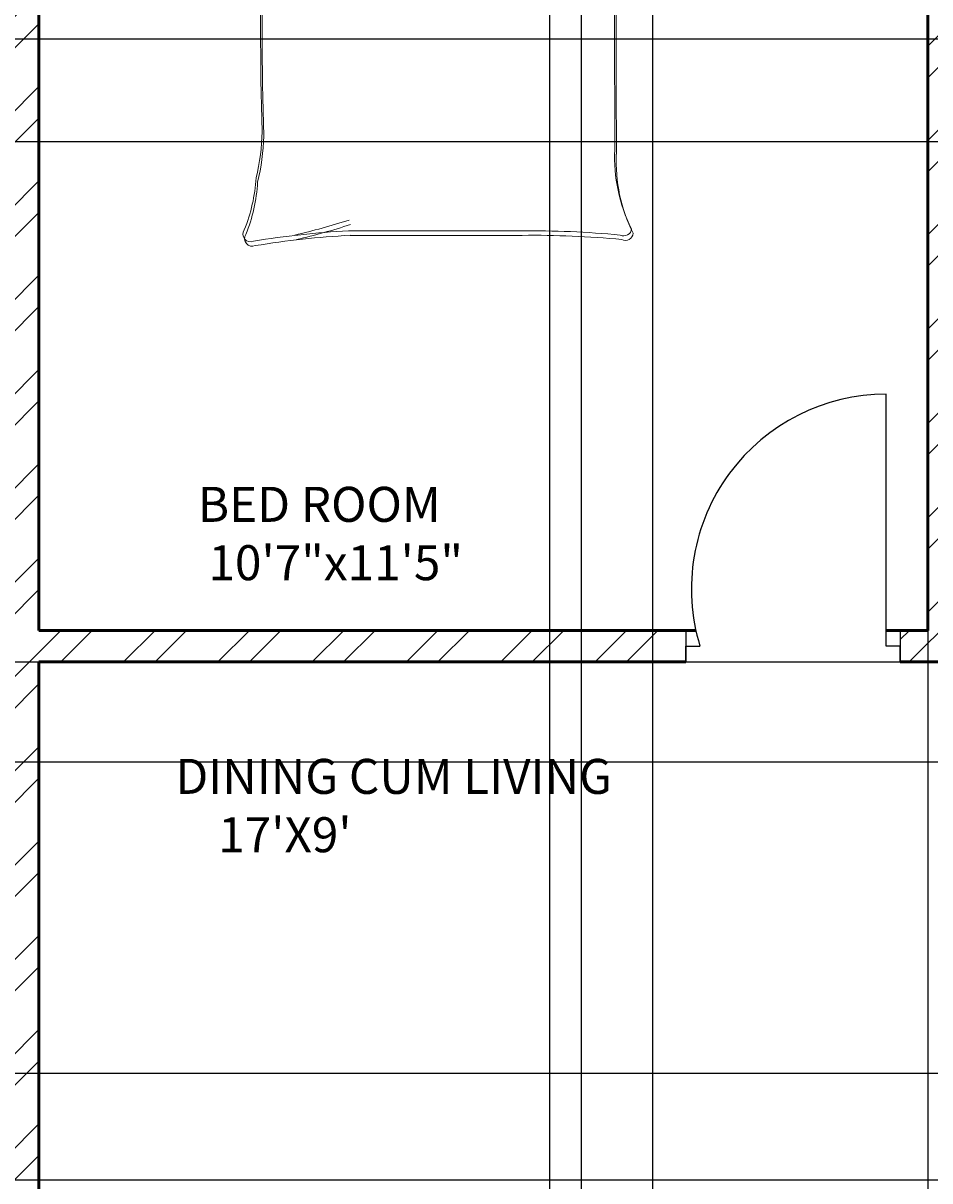
# Model space of a CAD drawing. Units: inches. Extents: x 2310 to 2937, y 1113 to 2410.
# Tile 20 of 23: x 2609 to 2739, y 2132 to 2297. Entities that reach past the tile are written whole.
import ezdxf

# ---------------------------------------------------------------- set-up
doc = ezdxf.new("R2010")
doc.units = ezdxf.units.IN
for name, color, linetype, lineweight in [('A-ANNO-DIMS', 2, 'Continuous', 18), ('A-AREA-IDEN', 7, 'Continuous', 18), ('A-DOOR', 31, 'Continuous', 25), ('A-FURN', 8, 'Continuous', 18), ('A-WALL', 7, 'Continuous', 50), ('A-WALL-PATT', 85, 'Continuous', 13)]:
    doc.layers.add(name, color=color, linetype=linetype, lineweight=lineweight)
doc.styles.get("Standard").update_dxf_attribs({"font": 'arial.ttf'})
doc.dimstyles.get("Standard").update_dxf_attribs({"dimtxt": 0.18, "dimasz": 0.18, "dimexe": 0.18, "dimexo": 0.0625, "dimgap": 0.09, "dimtad": 0, "dimtih": 1, "dimtoh": 1, "dimdec": 4, "dimzin": 0, "dimdsep": 46, "dimtxsty": 'Standard', "dimcen": 0.09, "dimadec": 0, "dimazin": 0, "dimtfac": 1, "dimtdec": 4, "dimtofl": 0, "dimtmove": 0, "dimatfit": 3, "dimfxl": 1, "dimtolj": 1, "dimtzin": 0, "dimarcsym": 0})

# ---------------------------------------------------------------- blocks, each defined once
blk = doc.blocks.new('BED-DOUBLE')
for p, q in [((3.56, 63.44), (3.56, 81.55)), ((3.56, 63.44), (3.56, 81.55)), ((3.56, 81.55), (51.58, 81.55)), ((51.35, 81.55), (51.35, 54.94)), ((51.35, 81.55), (51.35, 54.94)), ((51.58, 81.55), (51.58, 80.91)), ((3.56, 80.01), (51.35, 80.01)), ((3.56, 80.01), (51.35, 80.01)), ((3.79, 62.8), (3.79, 80.91)), ((3.79, 62.8), (3.79, 80.91)), ((24.62, 79.1), (26.07, 79.68)), ((24.62, 79.1), (26.07, 79.68)), ((26.07, 79.68), (26.65, 74.33)), ((26.07, 79.68), (26.65, 74.33)), ((51.58, 80.91), (51.58, 54.3)), ((51.58, 80.91), (51.58, 54.3)), ((3.79, 79.38), (51.58, 79.38)), ((3.79, 79.38), (51.58, 79.38)), ((3.98, 78.21), (8.27, 78.54)), ((3.98, 78.23), (4.56, 75.05)), ((3.98, 78.23), (4.56, 75.05)), ((3.99, 78.21), (8.27, 78.54)), ((4.21, 77.57), (8.49, 77.9)), ((4.21, 77.57), (8.49, 77.9)), ((8.27, 78.54), (8.37, 78.52)), ((8.27, 78.54), (8.37, 78.52)), ((8.37, 78.52), (12.19, 78.23)), ((8.37, 78.52), (12.19, 78.23)), ((8.49, 77.9), (8.6, 77.88)), ((8.49, 77.9), (8.6, 77.88)), ((8.6, 77.88), (12.42, 77.59)), ((8.6, 77.88), (12.42, 77.59)), ((12.19, 78.23), (17.69, 77.22)), ((12.19, 78.23), (17.69, 77.22)), ((14.94, 77.8), (16.97, 78.52)), ((14.94, 77.8), (16.96, 78.52)), ((15.17, 77.16), (17.19, 77.88)), ((15.17, 77.16), (17.19, 77.88)), ((16.96, 78.52), (19.86, 79.24)), ((16.97, 78.52), (19.86, 79.24)), ((17.19, 77.88), (20.08, 78.61)), ((17.19, 77.88), (20.08, 78.61)), ((19.86, 79.24), (20.18, 79.24)), ((19.86, 79.24), (20.18, 79.24)), ((20.08, 78.61), (20.41, 78.61)), ((20.08, 78.61), (20.41, 78.61)), ((20.18, 79.24), (24.62, 79.1)), ((20.18, 79.24), (24.62, 79.1)), ((20.41, 78.61), (24.85, 78.46)), ((20.41, 78.61), (24.85, 78.46)), ((24.85, 78.46), (26.3, 79.04)), ((24.85, 78.46), (26.3, 79.04)), ((26.3, 79.04), (26.88, 73.69)), ((26.3, 79.04), (26.88, 73.69)), ((28.06, 79.06), (27.82, 73.68)), ((28.06, 79.06), (27.82, 73.68)), ((28.29, 78.42), (28.05, 73.04)), ((28.29, 78.42), (28.05, 73.04)), ((29.54, 78.57), (28.06, 79.06)), ((29.54, 78.57), (28.06, 79.06)), ((29.77, 77.93), (28.29, 78.42)), ((29.77, 77.93), (28.29, 78.42)), ((33.97, 78.99), (29.54, 78.57)), ((33.97, 78.99), (29.54, 78.57)), ((34.2, 78.35), (29.77, 77.93)), ((34.2, 78.35), (29.77, 77.93)), ((34.29, 79.01), (33.97, 78.99)), ((34.29, 79.01), (33.97, 78.99)), ((34.52, 78.37), (34.2, 78.35)), ((34.52, 78.37), (34.2, 78.35)), ((37.22, 78.47), (34.29, 79.01)), ((37.22, 78.47), (34.29, 79.01)), ((37.45, 77.83), (34.52, 78.37)), ((37.45, 77.83), (34.52, 78.37)), ((42, 78.48), (36.58, 77.13)), ((42, 78.48), (36.58, 77.13)), ((42.23, 77.84), (36.81, 76.49)), ((42.23, 77.84), (36.81, 76.49)), ((39.29, 77.87), (37.22, 78.47)), ((39.29, 77.87), (37.22, 78.47)), ((39.52, 77.24), (37.45, 77.83)), ((39.51, 77.24), (37.45, 77.83)), ((45.8, 79.01), (42, 78.48)), ((45.8, 79.01), (42, 78.48)), ((46.03, 78.37), (42.23, 77.84)), ((46.03, 78.37), (42.23, 77.84)), ((50.2, 78.99), (44.8, 79.09)), ((44.8, 79.09), (45.8, 79.01)), ((50.2, 78.99), (44.8, 79.09)), ((44.8, 79.09), (45.8, 79.01)), ((50.43, 78.35), (45.02, 78.45)), ((45.02, 78.45), (46.03, 78.37)), ((50.43, 78.35), (45.02, 78.45)), ((45.02, 78.45), (46.03, 78.37)), ((50.2, 78.99), (49.82, 75.78)), ((50.2, 78.99), (49.82, 75.78)), ((50.43, 78.35), (50.05, 75.14)), ((50.43, 78.35), (50.05, 75.14)), ((4.21, 77.59), (4.79, 74.41)), ((4.21, 77.59), (4.79, 74.41)), ((12.42, 77.59), (17.92, 76.58)), ((12.42, 77.59), (17.92, 76.58)), ((4.56, 75.05), (4.13, 72.45)), ((4.56, 75.05), (4.13, 72.45)), ((5.14, 72.59), (6.15, 75.34)), ((5.14, 72.59), (6.15, 75.34)), ((5.37, 71.95), (6.38, 74.7)), ((5.37, 71.95), (6.38, 74.7)), ((49.4, 73.29), (48.21, 75.97)), ((49.4, 73.29), (48.21, 75.97)), ((49.62, 72.65), (48.44, 75.33)), ((49.62, 72.65), (48.44, 75.33)), ((49.82, 75.78), (50.42, 73.21)), ((49.82, 75.78), (50.41, 73.21)), ((50.05, 75.14), (50.64, 72.57)), ((50.05, 75.14), (50.64, 72.57)), ((4.79, 74.41), (4.35, 71.81)), ((4.79, 74.41), (4.35, 71.81)), ((26.65, 74.33), (27.23, 71.15)), ((26.65, 74.33), (27.23, 71.15)), ((26.88, 73.69), (27.45, 70.51)), ((26.88, 73.69), (27.45, 70.51)), ((27.82, 73.68), (27.44, 70.47)), ((27.82, 73.68), (27.44, 70.47)), ((28.05, 73.04), (27.67, 69.83)), ((28.05, 73.04), (27.67, 69.83)), ((50.2, 69.72), (49.4, 73.29)), ((50.2, 69.72), (49.4, 73.29)), ((50.42, 73.21), (49.9, 72.16)), ((50.41, 73.21), (49.9, 72.16)), ((4.13, 72.45), (4.7, 71.44)), ((4.13, 72.45), (4.7, 71.44)), ((4.35, 71.81), (4.93, 70.8)), ((4.35, 71.81), (4.93, 70.8)), ((4.56, 68.98), (5.14, 72.59)), ((4.56, 68.98), (5.14, 72.59)), ((4.79, 68.34), (5.37, 71.95)), ((4.79, 68.34), (5.37, 71.95)), ((27.23, 71.15), (27.23, 69.85)), ((27.23, 71.15), (27.23, 69.85)), ((50.43, 69.08), (49.62, 72.65)), ((50.43, 69.08), (49.62, 72.65)), ((50.64, 72.57), (50.13, 71.52)), ((50.64, 72.57), (50.13, 71.52)), ((27.23, 69.85), (26.65, 67.97)), ((27.23, 69.85), (26.65, 67.97)), ((27.44, 70.47), (27.52, 69.17)), ((27.44, 70.47), (27.52, 69.17)), ((27.45, 70.51), (27.45, 69.21)), ((27.45, 70.51), (27.45, 69.21)), ((27.67, 69.83), (27.75, 68.53)), ((27.67, 69.83), (27.75, 68.53)), ((50.01, 68.11), (50.2, 69.72)), ((50.01, 68.11), (50.2, 69.72)), ((4.85, 67.39), (4.56, 68.98)), ((4.85, 67.39), (4.56, 68.98)), ((5.08, 66.75), (4.79, 68.34)), ((5.08, 66.75), (4.79, 68.34)), ((26.65, 67.97), (26.65, 65.29)), ((26.65, 67.97), (26.65, 65.29)), ((27.45, 69.21), (26.88, 67.33)), ((27.45, 69.21), (26.88, 67.33)), ((27.52, 69.17), (28.22, 67.33)), ((27.52, 69.17), (28.22, 67.33)), ((27.75, 68.53), (28.45, 66.69)), ((27.75, 68.53), (28.44, 66.69)), ((50.78, 64.98), (50.01, 68.11)), ((50.78, 64.98), (50.01, 68.11)), ((50.24, 67.48), (50.43, 69.08)), ((50.24, 67.48), (50.43, 69.08)), ((4.27, 64.21), (4.85, 67.39)), ((4.27, 64.21), (4.85, 67.39)), ((4.5, 63.57), (5.08, 66.75)), ((4.5, 63.57), (5.08, 66.75)), ((24.19, 65.29), (21.04, 66.38)), ((24.19, 65.29), (21.05, 66.38)), ((26.88, 67.33), (26.88, 64.65)), ((26.88, 67.33), (26.88, 64.65)), ((28.22, 67.33), (28.38, 64.66)), ((28.22, 67.33), (28.38, 64.66)), ((28.44, 66.69), (28.61, 64.02)), ((28.45, 66.69), (28.61, 64.02)), ((51.01, 64.34), (50.24, 67.48)), ((51.01, 64.34), (50.24, 67.48)), ((9.37, 64.93), (4.27, 64.21)), ((9.37, 64.93), (4.27, 64.21)), ((6.47, 65.92), (10.5, 65.25)), ((6.47, 65.92), (10.5, 65.25)), ((6.7, 65.28), (10.73, 64.61)), ((6.7, 65.28), (10.73, 64.61)), ((10.5, 65.25), (9.37, 64.93)), ((10.5, 65.25), (9.37, 64.93)), ((10.73, 64.61), (9.6, 64.29)), ((10.73, 64.61), (9.6, 64.29)), ((10.5, 65.25), (17.51, 64.82)), ((10.5, 65.25), (17.51, 64.82)), ((10.73, 64.61), (17.74, 64.18)), ((10.73, 64.61), (17.74, 64.18)), ((17.51, 64.82), (19.47, 65.38)), ((17.51, 64.82), (19.47, 65.38)), ((17.74, 64.18), (19.7, 64.74)), ((17.74, 64.18), (19.7, 64.74)), ((19.47, 65.38), (24.6, 64.98)), ((19.47, 65.38), (24.6, 64.98)), ((19.7, 64.74), (24.83, 64.34)), ((19.7, 64.74), (24.83, 64.34)), ((24.42, 64.65), (21.27, 65.74)), ((24.42, 64.65), (21.27, 65.74)), ((26.65, 65.29), (24.19, 65.29)), ((26.65, 65.29), (24.19, 65.29)), ((26.88, 64.65), (24.42, 64.65)), ((26.88, 64.65), (24.42, 64.65)), ((28.38, 64.66), (30.84, 64.81)), ((28.38, 64.66), (30.84, 64.81)), ((30.84, 64.81), (33.91, 66.09)), ((30.84, 64.81), (33.91, 66.09)), ((31.06, 64.17), (34.14, 65.45)), ((31.07, 64.17), (34.14, 65.45)), ((32.65, 65.92), (36.68, 65.25)), ((32.65, 65.92), (36.68, 65.25)), ((32.88, 65.28), (36.91, 64.61)), ((32.88, 65.28), (36.91, 64.61)), ((36.68, 65.25), (43.69, 64.82)), ((36.68, 65.25), (43.69, 64.82)), ((36.91, 64.61), (43.92, 64.18)), ((36.91, 64.61), (43.92, 64.18)), ((43.69, 64.82), (45.65, 65.38)), ((43.69, 64.82), (45.65, 65.38)), ((43.92, 64.18), (45.88, 64.74)), ((43.92, 64.18), (45.88, 64.74)), ((45.65, 65.38), (50.78, 64.98)), ((45.65, 65.38), (50.78, 64.98)), ((45.88, 64.74), (51.01, 64.34)), ((45.88, 64.74), (51.01, 64.34)), ((9.6, 64.29), (4.5, 63.57)), ((9.6, 64.29), (4.5, 63.57)), ((28.61, 64.02), (31.07, 64.17)), ((28.61, 64.02), (31.06, 64.17)), ((30.35, 64.17), (34.54, 57.67)), ((30.35, 64.17), (34.54, 57.67)), ((30.57, 63.53), (34.76, 57.03)), ((30.57, 63.53), (34.76, 57.03)), ((40.73, 61.23), (32.39, 64.17)), ((40.73, 61.23), (32.39, 64.17)), ((40.96, 60.59), (32.62, 63.53)), ((40.96, 60.59), (32.62, 63.53)), ((46.31, 59.22), (40.73, 61.23)), ((46.31, 59.22), (40.73, 61.23)), ((46.53, 58.58), (40.96, 60.59)), ((46.53, 58.58), (40.96, 60.59)), ((49.25, 57.05), (46.31, 59.22)), ((49.25, 57.05), (46.31, 59.22)), ((49.48, 56.41), (46.53, 58.58)), ((49.48, 56.41), (46.53, 58.58)), ((34.54, 57.67), (36.24, 53.18)), ((34.54, 57.67), (36.24, 53.18)), ((34.76, 57.03), (36.47, 52.54)), ((34.76, 57.03), (36.47, 52.54)), ((52.95, 53.8), (49.25, 57.05)), ((52.95, 53.8), (49.25, 57.05)), ((53.18, 53.16), (49.48, 56.41)), ((53.18, 53.16), (49.48, 56.41)), ((36.24, 53.18), (36.55, 51.17)), ((36.24, 53.18), (36.55, 51.17)), ((41.04, 52.72), (44.45, 53.18)), ((41.04, 52.72), (44.45, 53.18)), ((44.45, 53.18), (48.32, 53.49)), ((44.45, 53.18), (48.32, 53.49)), ((48.32, 53.49), (51.42, 53.18)), ((48.32, 53.49), (51.42, 53.18)), ((51.42, 53.18), (52.95, 53.8)), ((51.42, 53.18), (52.95, 53.8)), ((51.65, 52.54), (53.18, 53.16)), ((51.65, 52.54), (53.18, 53.16)), ((53.03, 52.06), (52.95, 53.8, 3.87)), ((53.03, 52.06), (52.95, 53.8, 3.87)), ((53.26, 51.42), (53.18, 53.16, 3.87)), ((53.26, 51.42), (53.18, 53.16, 3.87)), ((36.47, 52.54), (36.78, 50.53)), ((36.47, 52.54), (36.78, 50.53)), ((36.55, 51.17), (39.03, 51.79)), ((36.55, 51.17), (39.03, 51.79)), ((39.03, 51.79), (41.04, 52.72)), ((39.03, 51.79), (41.04, 52.72)), ((39.26, 51.15), (41.27, 52.08)), ((39.26, 51.15), (41.27, 52.08)), ((41.27, 52.08), (44.68, 52.54)), ((41.27, 52.08), (44.68, 52.54)), ((44.68, 52.54), (48.55, 52.85)), ((44.68, 52.54), (48.55, 52.85)), ((48.55, 52.85), (51.65, 52.54)), ((48.55, 52.85), (51.65, 52.54)), ((36.78, 50.53), (39.26, 51.15)), ((36.78, 50.53), (39.26, 51.15)), ((15.15, 2.3), (39.76, 2.3)), ((15.15, 2.3), (39.76, 2.3)), ((15.38, 1.66), (39.99, 1.66)), ((15.38, 1.66), (39.99, 1.66))]:
    blk.add_line(p, q)
for centre, radius, start, end in [((85.25, 61.45), 83.31, 178.7218, 185.604), ((85.25, 61.45), 83.31, 178.7218, 185.604), ((21.45, -100.5), 164.97, 86.0865, 96.7821), ((21.45, -100.5), 164.97, 86.0865, 96.7821), ((21.67, -101.14), 164.97, 86.0865, 96.7821), ((21.67, -101.14), 164.97, 86.0865, 96.7821), ((85.48, 60.81), 83.31, 178.7218, 185.604), ((85.48, 60.81), 83.31, 178.7218, 185.604), ((17.84, -74.77), 129.02, 81.7845, 96.9006), ((17.84, -74.77), 129.02, 81.7845, 96.9006), ((18.07, -75.41), 129.02, 81.7845, 96.9006), ((18.07, -75.41), 129.02, 81.7845, 96.9006), ((-167.22, 50.37), 170.11, 358.4762, 1.0082), ((-167.22, 50.37), 170.11, 358.4762, 1.0082), ((-166.99, 49.74), 170.11, 358.4762, 1.0082), ((-166.99, 49.74), 170.11, 358.4762, 1.0082), ((31.24, 80.07), 29.65, 280.6617, 289.8806), ((31.24, 80.07), 29.65, 280.6617, 289.8806), ((31.47, 79.43), 29.65, 280.6617, 289.8806), ((31.47, 79.43), 29.65, 280.6617, 289.8806), ((43.83, 46.48), 6.22, 78.6608, 113.7384), ((43.83, 46.48), 6.22, 78.6608, 113.7384), ((44.06, 45.84), 6.22, 78.6608, 113.7384), ((44.06, 45.84), 6.22, 78.6608, 113.7384), ((51.41, 88.2), 36.18, 259.8763, 272.5657), ((51.41, 88.2), 36.18, 259.8763, 272.5657), ((51.64, 87.57), 36.18, 259.8763, 272.5657), ((51.64, 87.57), 36.18, 259.8763, 272.5657), ((182.35, 45.23), 129.5, 176.9791, 183.8365), ((182.35, 45.23), 129.5, 176.9791, 183.8365), ((182.58, 44.59), 129.5, 176.9791, 183.8365), ((182.58, 44.59), 129.5, 176.9791, 183.8365), ((36.72, 51.11), 0.185, 160.2464, 271.1377), ((36.72, 51.11), 0.185, 160.2464, 271.1377), ((36.95, 50.47), 0.185, 160.2464, 271.1377), ((36.95, 50.47), 0.185, 160.2464, 271.1377), ((484.91, 30.93), 482.31, 178.2277, 181.7185), ((484.91, 30.93), 482.31, 178.2277, 181.7185), ((485.14, 30.3), 482.31, 178.2277, 181.7185), ((485.14, 30.3), 482.31, 178.2277, 181.7185), ((-4508.66, 13.73), 4561.86, 0.00217, 0.28689), ((-4508.66, 13.73), 4561.86, 0.00217, 0.28689), ((-4508.43, 13.09), 4561.86, 0.00217, 0.28689), ((-4508.43, 13.09), 4561.86, 0.00217, 0.28689), ((-26.81, 17.03), 29.63, 346.0648, 358.9113), ((-26.81, 17.03), 29.63, 346.0648, 358.9113), ((-26.58, 16.39), 29.63, 346.0648, 358.9113), ((-26.58, 16.39), 29.63, 346.0648, 358.9113), ((76.24, 12.88), 23.07, 177.4714, 206.4681), ((76.24, 12.88), 23.07, 177.4714, 206.4681), ((76.47, 12.24), 23.07, 177.4714, 206.4681), ((76.47, 12.24), 23.07, 177.4714, 206.4681), ((-21.57, 11.27), 23.56, 337.9751, 356.652), ((-21.57, 11.27), 23.56, 337.9751, 356.652), ((-21.34, 10.63), 23.56, 337.9751, 356.652), ((-21.34, 10.63), 23.56, 337.9751, 356.652), ((-17.14, 105.26), 106.46, 283.3832, 287.7053), ((-17.14, 105.26), 106.46, 283.3832, 287.7053), ((1.17, 1.83), 1.09, 146.1736, 293.4781), ((1.17, 1.83), 1.09, 146.1736, 293.4781), ((1.4, 1.19), 1.09, 146.1736, 293.4781), ((1.4, 1.19), 1.09, 146.1736, 293.4781), ((21.51, -119.29), 121.76, 92.9958, 99.4091), ((21.51, -119.29), 121.76, 92.9958, 99.4091), ((21.74, -119.93), 121.76, 92.9958, 99.4091), ((21.74, -119.93), 121.76, 92.9958, 99.4091), ((-16.91, 104.62), 106.46, 283.3832, 287.7053), ((-16.91, 104.62), 106.46, 283.3832, 287.7053), ((41.24, -130.73), 133.04, 84.4998, 90.6351), ((41.24, -130.73), 133.04, 84.4998, 90.6351), ((41.47, -131.37), 133.04, 84.4998, 90.6351), ((41.47, -131.37), 133.04, 84.4998, 90.6351), ((54.5, 2.68), 1.1, 242.6588, 356.02), ((54.5, 2.68), 1.1, 242.6588, 356.02), ((54.72, 2.04), 1.1, 242.6588, 356.02), ((54.72, 2.04), 1.1, 242.6588, 356.02)]:
    blk.add_arc(centre, radius, start, end)
blk = doc.blocks.new('*D42')
at = {"layer": 'A-ANNO-DIMS', "color": 0, "lineweight": -2, "transparency": 16777216}
for p, q in [((2699.14, 2347.45), (2699.14, 1649.5)), ((2738.49, 2347.45), (2738.49, 1649.5)), ((2699.32, 1649.68), (2718.42, 1649.68)), ((2738.31, 1649.68), (2719.21, 1649.68))]:
    blk.add_line(p, q, dxfattribs=at)
at = {"layer": 'A-ANNO-DIMS', "color": 0, "transparency": 16777216}
for points in [[(2699.32, 1649.71), (2699.32, 1649.65), (2699.14, 1649.68)], [(2738.31, 1649.71), (2738.31, 1649.65), (2738.49, 1649.68)]]:
    blk.add_solid(points, dxfattribs=at)
at = {"layer": 'Defpoints', "color": 0, "transparency": 16777216}
for p in [(2699.14, 2347.51), (2738.49, 2347.51), (2738.49, 1649.68)]:
    blk.add_point(p, dxfattribs=at)
at = {"layer": 'A-ANNO-DIMS', "color": 0, "transparency": 16777216, "insert": (2718.81, 1649.68), "char_height": 0.18, "attachment_point": 5}
blk.add_mtext('\\A1;39.35', dxfattribs=at)
blk = doc.blocks.new('*D53')
at = {"layer": 'A-ANNO-DIMS', "color": 0, "lineweight": -2, "transparency": 16777216}
for p, q in [((2403.55, 2295.01), (2858.02, 2295.01)), ((2857.84, 2294.83), (2857.84, 2287.87)), ((2857.84, 2280.55), (2857.84, 2287.51)), ((2403.55, 2280.37), (2858.02, 2280.37))]:
    blk.add_line(p, q, dxfattribs=at)
at = {"layer": 'A-ANNO-DIMS', "color": 0, "transparency": 16777216}
for points in [[(2857.81, 2294.83), (2857.87, 2294.83), (2857.84, 2295.01)], [(2857.81, 2280.55), (2857.87, 2280.55), (2857.84, 2280.37)]]:
    blk.add_solid(points, dxfattribs=at)
at = {"layer": 'Defpoints', "color": 0, "transparency": 16777216}
for p in [(2403.49, 2295.01), (2403.49, 2280.37), (2857.84, 2280.37)]:
    blk.add_point(p, dxfattribs=at)
at = {"layer": 'A-ANNO-DIMS', "color": 0, "transparency": 16777216, "insert": (2857.84, 2287.69), "char_height": 0.18, "attachment_point": 5}
blk.add_mtext('\\A1;14.644', dxfattribs=at)
blk = doc.blocks.new('*D54')
at = {"layer": 'A-ANNO-DIMS', "color": 0, "lineweight": -2, "transparency": 16777216}
for p, q in [((2403.55, 2206.01), (2858.02, 2206.01)), ((2857.84, 2205.83), (2857.84, 2199.07)), ((2857.84, 2191.94), (2857.84, 2198.7)), ((2403.55, 2191.76), (2858.02, 2191.76))]:
    blk.add_line(p, q, dxfattribs=at)
at = {"layer": 'A-ANNO-DIMS', "color": 0, "transparency": 16777216}
for points in [[(2857.81, 2205.83), (2857.87, 2205.83), (2857.84, 2206.01)], [(2857.81, 2191.94), (2857.87, 2191.94), (2857.84, 2191.76)]]:
    blk.add_solid(points, dxfattribs=at)
at = {"layer": 'Defpoints', "color": 0, "transparency": 16777216}
for p in [(2403.49, 2206.01), (2403.49, 2191.76), (2857.84, 2191.76)]:
    blk.add_point(p, dxfattribs=at)
at = {"layer": 'A-ANNO-DIMS', "color": 0, "transparency": 16777216, "insert": (2857.84, 2198.89), "char_height": 0.18, "attachment_point": 5}
blk.add_mtext('\\A1;14.255', dxfattribs=at)
blk = doc.blocks.new('*D68')
at = {"layer": 'A-ANNO-DIMS', "color": 0, "lineweight": -2, "transparency": 16777216}
for p, q in [((2684.49, 1999.58), (2684.49, 2390.54)), ((2684.67, 2390.36), (2686.48, 2390.36)), ((2688.81, 2390.36), (2686.99, 2390.36)), ((2688.99, 1999.58), (2688.99, 2390.54))]:
    blk.add_line(p, q, dxfattribs=at)
at = {"layer": 'A-ANNO-DIMS', "color": 0, "transparency": 16777216}
for points in [[(2684.67, 2390.39), (2684.67, 2390.33), (2684.49, 2390.36)], [(2688.81, 2390.39), (2688.81, 2390.33), (2688.99, 2390.36)]]:
    blk.add_solid(points, dxfattribs=at)
at = {"layer": 'Defpoints', "color": 0, "transparency": 16777216}
for p in [(2688.99, 2390.36), (2684.49, 1999.51), (2688.99, 1999.51)]:
    blk.add_point(p, dxfattribs=at)
at = {"layer": 'A-ANNO-DIMS', "color": 0, "transparency": 16777216, "insert": (2686.74, 2390.36), "char_height": 0.18, "attachment_point": 5}
blk.add_mtext('\\A1;4.5', dxfattribs=at)
blk = doc.blocks.new('*D70')
at = {"layer": 'A-ANNO-DIMS', "color": 0, "lineweight": -2, "transparency": 16777216}
for p, q in [((2475.96, 2147.28), (2858.02, 2147.28)), ((2857.84, 2147.1), (2857.84, 2139.83)), ((2857.84, 2132.2), (2857.84, 2139.47)), ((2475.96, 2132.02), (2858.02, 2132.02))]:
    blk.add_line(p, q, dxfattribs=at)
at = {"layer": 'A-ANNO-DIMS', "color": 0, "transparency": 16777216}
for points in [[(2857.81, 2147.1), (2857.87, 2147.1), (2857.84, 2147.28)], [(2857.81, 2132.2), (2857.87, 2132.2), (2857.84, 2132.02)]]:
    blk.add_solid(points, dxfattribs=at)
at = {"layer": 'Defpoints', "color": 0, "transparency": 16777216}
for p in [(2475.89, 2147.28), (2857.84, 2147.28), (2475.89, 2132.02)]:
    blk.add_point(p, dxfattribs=at)
at = {"layer": 'A-ANNO-DIMS', "color": 0, "transparency": 16777216, "insert": (2857.84, 2139.65), "char_height": 0.18, "attachment_point": 5}
blk.add_mtext('\\A1;15.257', dxfattribs=at)

msp = doc.modelspace()

# ---------------------------------------------------------------- hatches: boundary and pattern name
at = {"layer": 'A-WALL-PATT'}
h = msp.add_hatch(dxfattribs=at)
h.set_pattern_fill('ANSI32', color=256)
h.paths.add_polyline_path([(2639.1394, 2356.5139), (2563.662, 2356.5139), (2563.662, 2347.5139), (2606.9859, 2347.5139), (2606.9859, 2210.5139), (2514.2692, 2210.5139), (2514.2692, 2206.0139), (2606.9859, 2206.0139), (2606.9859, 2098.0139), (2602.689, 2098.0139), (2602.689, 2093.5139), (2615.5262, 2093.5139), (2615.5262, 2095.7639), (2615.5262, 2098.0139), (2611.4859, 2098.0139), (2611.4859, 2206.0139), (2703.9391, 2206.0139), (2703.9391, 2208.2639), (2703.9391, 2210.5139), (2611.4859, 2210.5139), (2611.4859, 2347.5139), (2639.1394, 2347.5139)])
h.paths.add_polyline_path([(2823.9859, 2356.5139), (2699.1394, 2356.5139), (2699.1394, 2347.5139), (2738.4859, 2347.5139), (2738.4859, 2343.9266), (2742.9859, 2343.9266), (2742.9859, 2347.5139), (2814.9859, 2347.5139), (2814.9859, 2336.76), (2823.9859, 2336.76)])
h.paths.add_polyline_path([(2823.9859, 2312.76), (2814.9859, 2312.76), (2814.9859, 2299.5139), (2742.9859, 2299.5139), (2742.9859, 2323.0159), (2740.7359, 2323.0159), (2738.4859, 2323.0159), (2738.4859, 2210.5139), (2734.5483, 2210.5139), (2734.5483, 2206.0139), (2746.8769, 2206.0139), (2746.8769, 2208.2639), (2746.8769, 2210.5139), (2742.9859, 2210.5139), (2742.9859, 2295.0139), (2814.9859, 2295.0139), (2814.9859, 2269.8977), (2823.9859, 2269.8977)])
h.paths.add_polyline_path([(2823.9859, 2210.5139), (2823.9859, 2233.8977), (2819.4859, 2233.8977), (2814.9859, 2233.8977), (2814.9859, 2210.5139), (2769.9745, 2210.5139), (2769.9745, 2206.0139), (2814.9859, 2206.0139), (2814.9859, 2178.3027), (2823.9859, 2178.3027)])
h.paths.add_polyline_path([(2823.9859, 2118.3027), (2819.4859, 2118.3027), (2814.9859, 2118.3027), (2814.9859, 2098.0139), (2647.0333, 2098.0139), (2647.0333, 2093.5139), (2814.9859, 2093.5139), (2814.9859, 1999.5139), (2650.6052, 1999.5139), (2650.6052, 1995.0139), (2814.9859, 1995.0139), (2814.9859, 1969.9784), (2823.9859, 1969.9784)])
h.paths.add_polyline_path([(2403.4859, 2093.5139), (2569.9888, 2093.5139), (2569.9888, 2095.7639), (2569.9888, 2098.0139), (2403.4859, 2098.0139), (2403.4859, 2131.7587), (2394.4859, 2131.7587), (2394.4859, 1967.522), (2403.4859, 1967.522), (2403.4859, 1995.0139), (2569.8903, 1995.0139), (2569.8903, 1997.2639), (2569.8903, 1999.5139), (2403.4859, 1999.5139)])
h.paths.add_polyline_path([(2503.662, 2356.5139), (2394.4859, 2356.5139), (2394.4859, 2337.9231), (2398.9859, 2337.9231), (2403.4859, 2337.9231), (2403.4859, 2347.5139), (2475.4859, 2347.5139), (2475.4859, 2343.0384), (2479.9859, 2343.0384), (2479.9859, 2347.5139), (2503.662, 2347.5139)])
h.paths.add_polyline_path([(2498.3065, 1745.5139), (2479.9859, 1745.5139), (2479.9859, 1749.1663), (2477.7359, 1749.1663), (2475.4859, 1749.1663), (2475.4859, 1745.5139), (2403.4859, 1745.5139), (2403.4859, 1753.6409), (2398.9859, 1753.6409), (2394.4859, 1753.6409), (2394.4859, 1736.5139), (2498.3065, 1736.5139), (2498.3065, 1741.0139)])
h.paths.add_polyline_path([(2479.9859, 1882.5139), (2483.9367, 1882.5139), (2483.9367, 1887.0139), (2471.5501, 1887.0139), (2471.5501, 1885.1969), (2471.5501, 1882.5139), (2475.4859, 1882.5139), (2475.4859, 1798.0139), (2403.4859, 1798.0139), (2403.4859, 1828.0433), (2402.2852, 1828.0433), (2394.4859, 1828.0433), (2394.4859, 1777.6409), (2403.4859, 1777.6409), (2403.4859, 1793.5139), (2475.4859, 1793.5139), (2475.4859, 1769.1696), (2479.9859, 1769.1696)])
h.paths.add_polyline_path([(2403.4859, 1907.522), (2398.9859, 1907.522), (2394.4859, 1907.522), (2394.4859, 1864.0433), (2403.4859, 1864.0433), (2403.4859, 1882.5139), (2448.9325, 1882.5139), (2448.9325, 1884.7639), (2448.9325, 1887.0139), (2403.4859, 1887.0139)])
h.paths.add_polyline_path([(2702.2061, 1887.0139), (2611.4859, 1887.0139), (2611.4859, 1995.0139), (2615.6132, 1995.0139), (2615.6132, 1999.5139), (2602.4798, 1999.5139), (2602.4798, 1997.2639), (2602.4798, 1995.0139), (2606.9859, 1995.0139), (2606.9859, 1887.0139), (2516.2443, 1887.0139), (2516.2443, 1884.7639), (2516.2443, 1882.5139), (2606.9859, 1882.5139), (2606.9859, 1745.5139), (2558.3065, 1745.5139), (2558.3065, 1736.5139), (2638.8921, 1736.5139), (2638.8921, 1741.0139), (2638.8921, 1745.5139), (2611.4859, 1745.5139), (2611.4859, 1882.5139), (2702.2061, 1882.5139)])
h.paths.add_polyline_path([(2823.9859, 1909.9784), (2819.4859, 1909.9784), (2814.9859, 1909.9784), (2814.9859, 1887.0139), (2769.144, 1887.0139), (2769.144, 1884.7639), (2769.144, 1882.5139), (2814.9859, 1882.5139), (2814.9859, 1854.1704), (2823.9859, 1854.1704)])
h.paths.add_polyline_path([(2823.9859, 1818.1704), (2819.4859, 1818.1704), (2814.9859, 1818.1704), (2814.9859, 1798.0139), (2742.9859, 1798.0139), (2742.9859, 1882.5139), (2746.805, 1882.5139), (2746.805, 1887.0139), (2733.7334, 1887.0139), (2733.7334, 1884.7639), (2733.7334, 1882.5139), (2738.4859, 1882.5139), (2738.4859, 1771.1728), (2740.7359, 1771.1728), (2742.9859, 1771.1728), (2742.9859, 1793.5139), (2814.9859, 1793.5139), (2814.9859, 1783.6684), (2823.9859, 1783.6684)])
h.paths.add_polyline_path([(2823.9859, 1759.6684), (2814.9859, 1759.6684), (2814.9859, 1745.5139), (2742.9859, 1745.5139), (2742.9859, 1748.9831), (2740.7359, 1748.9831), (2738.4859, 1748.9831), (2738.4859, 1745.5139), (2698.8921, 1745.5139), (2698.8921, 1736.5139), (2823.9859, 1736.5139)])

# ---------------------------------------------------------------- linework, layer by layer
at = {"layer": 'A-DOOR'}
for p, q in [((2732.5483, 2208.2639), (2732.5483, 2244.2639)), ((2703.9391, 2210.5139), (2703.9391, 2206.0139)), ((2734.5483, 2210.5139), (2734.5483, 2206.0139)), ((2703.9391, 2206.0139), (2703.9391, 2208.2639)), ((2703.9391, 2208.2639), (2705.9391, 2208.2639)), ((2734.5483, 2208.2639), (2732.5483, 2208.2639)), ((2734.5483, 2206.0139), (2734.5483, 2208.2639))]:
    msp.add_line(p, q, dxfattribs=at)
msp.add_arc((2732.5483, 2216.4299), 27.834, 90, 197.060528, dxfattribs=at)
at = {"layer": 'A-WALL'}
for p, q in [((2611.4859, 2347.5139), (2611.4859, 2210.5139)), ((2738.4859, 2323.0159), (2738.4859, 2210.5139)), ((2611.4859, 2210.5139), (2705.3503, 2210.5139)), ((2732.5483, 2210.5139), (2738.4859, 2210.5139)), ((2611.4859, 2206.0139), (2703.9391, 2206.0139)), ((2611.4859, 2206.0139), (2611.4859, 2098.0139)), ((2734.5483, 2206.0139), (2746.8769, 2206.0139))]:
    msp.add_line(p, q, dxfattribs=at)

# ---------------------------------------------------------------- block references
at = {"layer": 'A-FURN'}
msp.add_blockref('BED-DOUBLE', (2640.5618, 2265.2919), dxfattribs=at)

# ---------------------------------------------------------------- texts
at = {"layer": 'A-AREA-IDEN', "char_height": 5, "attachment_point": 1}
for s, width, insert in [('        BED ROOM\\P         10\'7"x11\'5"', 95.729576, (2621.9594, 2231.0292)), ("      DINING CUM LIVING\\P          17'X9'", 162.884669, (2621.8269, 2192.1703))]:
    msp.add_mtext_dynamic_manual_height_columns(s, width=width, gutter_width=12.5, heights=[0], dxfattribs=dict(at, insert=insert))

# ---------------------------------------------------------------- dimensions: what is measured, and where the dimension line sits
at = {"layer": 'A-ANNO-DIMS'}
for base, p1, p2, override, picture, middle in [((2688.9859, 2390.3639), (2684.4859, 1999.5139), (2688.9859, 1999.5139), {"dimdec": 1, "dimlfac": 1, "dimrnd": 0, "dimzin": 0, "dimdsep": 46, "dimlunit": 2}, '*D68', (2686.7359, 2390.3639)), ((2738.4859, 1649.6807), (2699.1394, 2347.5139), (2738.4859, 2347.5139), {"dimdec": 2, "dimlfac": 1, "dimrnd": 0, "dimzin": 0, "dimdsep": 46, "dimlunit": 2}, '*D42', (2718.8127, 1649.6807))]:
    dim = msp.add_linear_dim(base=base, p1=p1, p2=p2, dimstyle='Standard', override=override, dxfattribs=at)
    dim.commit()
    dim.dimension.update_dxf_attribs({"geometry": picture, "text_midpoint": middle})
for base, p1, p2, picture, middle in [((2857.8359, 2280.3697), (2403.4859, 2295.0139), (2403.4859, 2280.3697), '*D53', (2857.8359, 2287.6918)), ((2857.8359, 2191.7587), (2403.4859, 2206.0139), (2403.4859, 2191.7587), '*D54', (2857.8359, 2198.8863)), ((2857.8359, 2147.2815), (2475.8929, 2132.0241), (2475.8929, 2147.2815), '*D70', (2857.8359, 2139.6528))]:
    dim = msp.add_linear_dim(base=base, p1=p1, p2=p2, angle=90, dimstyle='Standard', override={"dimdec": 3, "dimlfac": 1, "dimrnd": 0, "dimzin": 0, "dimdsep": 46, "dimlunit": 2}, dxfattribs=at)
    dim.commit()
    dim.dimension.update_dxf_attribs({"geometry": picture, "text_midpoint": middle})

doc.saveas('drawing.dxf')
